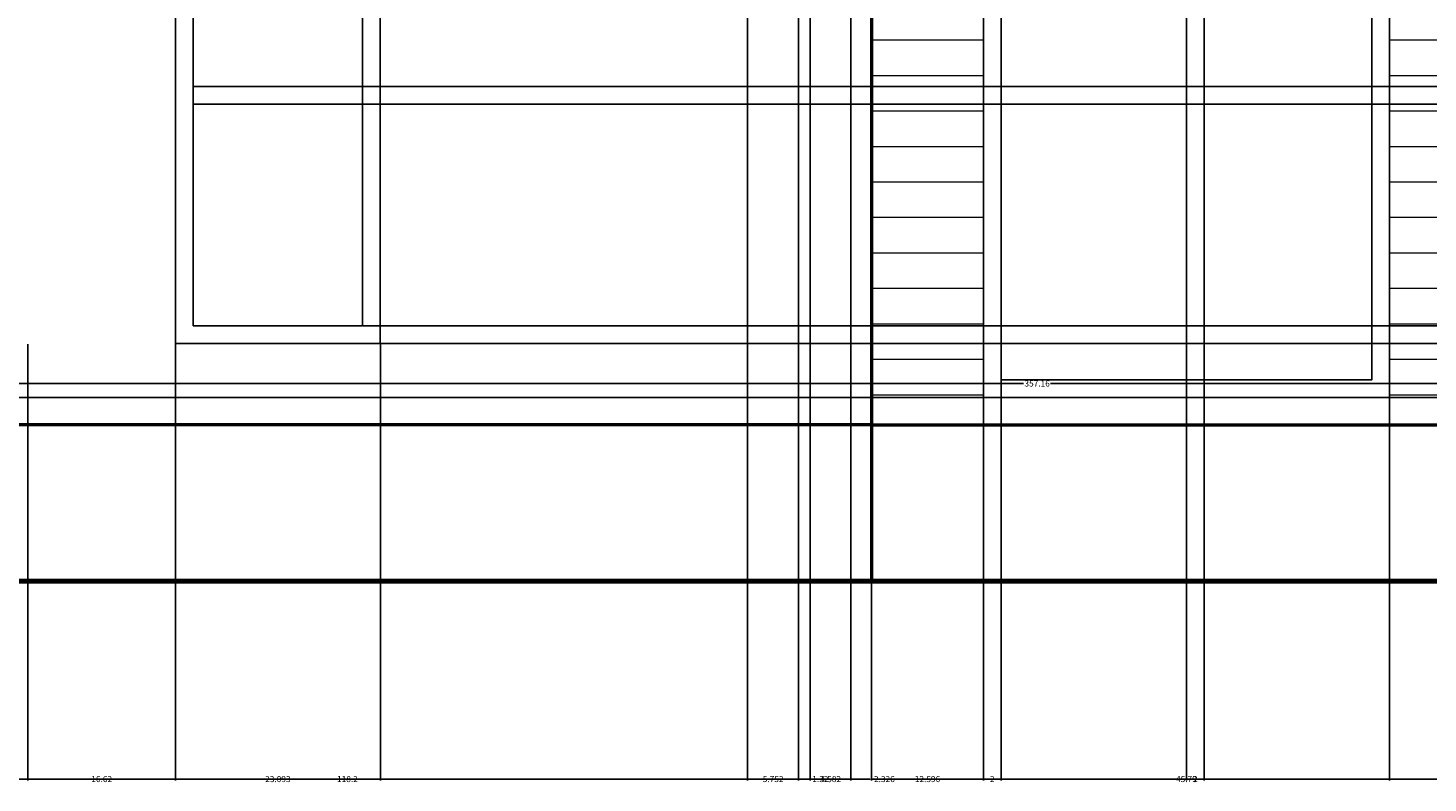
# Model space of a CAD drawing. Units: inches. Extents: x -139 to 346, y 72 to 413.
# Tile 3 of 18: x 18 to 175, y 72 to 157. Entities that reach past the tile are written whole.
import ezdxf

# ---------------------------------------------------------------- set-up
doc = ezdxf.new("R2010")
doc.units = ezdxf.units.IN
doc.header["$MEASUREMENT"] = 0
for name, color, linetype, lineweight in [('A-ANNO-DIMS', 2, 'Continuous', 18), ('A-DOOR', 3, 'Continuous', 25), ('A-GLAZ', 4, 'Continuous', 25), ('A-WALL', 7, 'Continuous', 50), ('A-WALL-PATT', 8, 'Continuous', 13), ('C-TOPO', 7, 'Continuous', 70)]:
    doc.layers.add(name, color=color, linetype=linetype, lineweight=lineweight)
doc.styles.get("Standard").update_dxf_attribs({"font": 'arial.ttf'})
doc.dimstyles.get("Standard").update_dxf_attribs({"dimtxt": 0.6875, "dimasz": 0.18, "dimexe": 0.18, "dimexo": 0.0625, "dimgap": 0.09, "dimtad": 0, "dimtih": 1, "dimtoh": 1, "dimdec": 4, "dimzin": 0, "dimdsep": 46, "dimlunit": 4, "dimtxsty": 'Standard', "dimcen": 0.09, "dimadec": 0, "dimazin": 0, "dimtfac": 1, "dimtdec": 4, "dimtofl": 0, "dimtmove": 0, "dimatfit": 3, "dimfxl": 1, "dimtolj": 1, "dimtzin": 0, "dimarcsym": 0})

# ---------------------------------------------------------------- blocks, each defined once
blk = doc.blocks.new('*D7')
at = {"layer": 'A-ANNO-DIMS', "color": 0, "lineweight": -2, "transparency": 16777216}
for p, q in [((-47.27, 95.04), (-47.27, 117.45)), ((-47.09, 117.27), (129.79, 117.27)), ((309.71, 117.27), (132.82, 117.27)), ((309.89, 95.04), (309.89, 117.45))]:
    blk.add_line(p, q, dxfattribs=at)
at = {"layer": 'A-ANNO-DIMS', "color": 0, "transparency": 16777216}
for points in [[(-47.09, 117.3), (-47.09, 117.24), (-47.27, 117.27)], [(309.71, 117.3), (309.71, 117.24), (309.89, 117.27)]]:
    blk.add_solid(points, dxfattribs=at)
at = {"layer": 'Defpoints', "color": 0, "transparency": 16777216}
for p in [(309.89, 117.27), (-47.27, 94.97), (309.89, 94.97)]:
    blk.add_point(p, dxfattribs=at)
at = {"layer": 'A-ANNO-DIMS', "color": 0, "transparency": 16777216, "insert": (131.31, 117.27), "char_height": 0.688, "attachment_point": 5}
blk.add_mtext('\\A1;357.16', dxfattribs=at)
blk = doc.blocks.new('*D10')
at = {"layer": 'A-ANNO-DIMS', "color": 0, "lineweight": -2, "transparency": 16777216}
for p, q in [((-5.54, 121.71), (-5.54, 72.49)), ((112.65, 112.54), (112.65, 72.49)), ((-5.36, 72.67), (52.34, 72.67)), ((112.47, 72.67), (54.77, 72.67))]:
    blk.add_line(p, q, dxfattribs=at)
at = {"layer": 'A-ANNO-DIMS', "color": 0, "transparency": 16777216}
for points in [[(-5.36, 72.7), (-5.36, 72.64), (-5.54, 72.67)], [(112.47, 72.7), (112.47, 72.64), (112.65, 72.67)]]:
    blk.add_solid(points, dxfattribs=at)
at = {"layer": 'Defpoints', "color": 0, "transparency": 16777216}
for p in [(-5.54, 121.78), (112.65, 112.6), (112.65, 72.67)]:
    blk.add_point(p, dxfattribs=at)
at = {"layer": 'A-ANNO-DIMS', "color": 0, "transparency": 16777216, "insert": (53.56, 72.67), "char_height": 0.688, "attachment_point": 5}
blk.add_mtext('\\A1;118.2', dxfattribs=at)
blk = doc.blocks.new('*D11')
at = {"layer": 'A-ANNO-DIMS', "color": 0, "lineweight": -2, "transparency": 16777216}
for p, q in [((112.65, 112.54), (112.65, 72.49)), ((309.89, 94.91), (309.89, 72.49)), ((112.83, 72.67), (209.79, 72.67)), ((309.71, 72.67), (212.75, 72.67))]:
    blk.add_line(p, q, dxfattribs=at)
at = {"layer": 'A-ANNO-DIMS', "color": 0, "transparency": 16777216}
for points in [[(112.83, 72.7), (112.83, 72.64), (112.65, 72.67)], [(309.71, 72.7), (309.71, 72.64), (309.89, 72.67)]]:
    blk.add_solid(points, dxfattribs=at)
at = {"layer": 'Defpoints', "color": 0, "transparency": 16777216}
for p in [(112.65, 112.6), (309.89, 94.97), (309.89, 72.67)]:
    blk.add_point(p, dxfattribs=at)
at = {"layer": 'A-ANNO-DIMS', "color": 0, "transparency": 16777216, "insert": (211.27, 72.67), "char_height": 0.688, "attachment_point": 5}
blk.add_mtext('\\A1;197.24', dxfattribs=at)
blk = doc.blocks.new('*D12')
at = {"layer": 'A-ANNO-DIMS', "color": 0, "lineweight": -2, "transparency": 16777216}
for p, q in [((-5.54, 121.71), (-5.54, 72.49)), ((17.55, 121.71), (17.55, 72.49)), ((-5.36, 72.67), (4.48, 72.67)), ((17.37, 72.67), (7.53, 72.67))]:
    blk.add_line(p, q, dxfattribs=at)
at = {"layer": 'A-ANNO-DIMS', "color": 0, "transparency": 16777216}
for points in [[(-5.36, 72.7), (-5.36, 72.64), (-5.54, 72.67)], [(17.37, 72.7), (17.37, 72.64), (17.55, 72.67)]]:
    blk.add_solid(points, dxfattribs=at)
at = {"layer": 'Defpoints', "color": 0, "transparency": 16777216}
for p in [(-5.54, 121.78), (17.55, 121.78), (17.55, 72.67)]:
    blk.add_point(p, dxfattribs=at)
at = {"layer": 'A-ANNO-DIMS', "color": 0, "transparency": 16777216, "insert": (6.01, 72.67), "char_height": 0.688, "attachment_point": 5}
blk.add_mtext('\\A1;23.093', dxfattribs=at)
blk = doc.blocks.new('*D13')
at = {"layer": 'A-ANNO-DIMS', "color": 0, "lineweight": -2, "transparency": 16777216}
for p, q in [((17.55, 121.71), (17.55, 72.49)), ((34.17, 121.71), (34.17, 72.49)), ((17.73, 72.67), (24.65, 72.67)), ((33.99, 72.67), (27.08, 72.67))]:
    blk.add_line(p, q, dxfattribs=at)
at = {"layer": 'A-ANNO-DIMS', "color": 0, "transparency": 16777216}
for points in [[(17.73, 72.7), (17.73, 72.64), (17.55, 72.67)], [(33.99, 72.7), (33.99, 72.64), (34.17, 72.67)]]:
    blk.add_solid(points, dxfattribs=at)
at = {"layer": 'Defpoints', "color": 0, "transparency": 16777216}
for p in [(17.55, 121.78), (34.17, 121.78), (34.17, 72.67)]:
    blk.add_point(p, dxfattribs=at)
at = {"layer": 'A-ANNO-DIMS', "color": 0, "transparency": 16777216, "insert": (25.86, 72.67), "char_height": 0.688, "attachment_point": 5}
blk.add_mtext('\\A1;16.62', dxfattribs=at)
blk = doc.blocks.new('*D14')
at = {"layer": 'A-ANNO-DIMS', "color": 0, "lineweight": -2, "transparency": 16777216}
for p, q in [((34.17, 121.71), (34.17, 72.49)), ((57.27, 121.71), (57.27, 72.49)), ((34.35, 72.67), (44.2, 72.67)), ((57.09, 72.67), (47.24, 72.67))]:
    blk.add_line(p, q, dxfattribs=at)
at = {"layer": 'A-ANNO-DIMS', "color": 0, "transparency": 16777216}
for points in [[(34.35, 72.7), (34.35, 72.64), (34.17, 72.67)], [(57.09, 72.7), (57.09, 72.64), (57.27, 72.67)]]:
    blk.add_solid(points, dxfattribs=at)
at = {"layer": 'Defpoints', "color": 0, "transparency": 16777216}
for p in [(34.17, 121.78), (57.27, 121.78), (57.27, 72.67)]:
    blk.add_point(p, dxfattribs=at)
at = {"layer": 'A-ANNO-DIMS', "color": 0, "transparency": 16777216, "insert": (45.72, 72.67), "char_height": 0.688, "attachment_point": 5}
blk.add_mtext('\\A1;23.093', dxfattribs=at)
blk = doc.blocks.new('*D15')
at = {"layer": 'A-ANNO-DIMS', "color": 0, "lineweight": -2, "transparency": 16777216}
for p, q in [((125.25, 115.61), (125.25, 72.49)), ((112.65, 112.54), (112.65, 72.49)), ((112.83, 72.67), (117.46, 72.67)), ((125.07, 72.67), (120.43, 72.67))]:
    blk.add_line(p, q, dxfattribs=at)
at = {"layer": 'A-ANNO-DIMS', "color": 0, "transparency": 16777216}
for points in [[(112.83, 72.7), (112.83, 72.64), (112.65, 72.67)], [(125.07, 72.7), (125.07, 72.64), (125.25, 72.67)]]:
    blk.add_solid(points, dxfattribs=at)
at = {"layer": 'Defpoints', "color": 0, "transparency": 16777216}
for p in [(125.25, 115.68), (112.65, 112.6), (125.25, 72.67)]:
    blk.add_point(p, dxfattribs=at)
at = {"layer": 'A-ANNO-DIMS', "color": 0, "transparency": 16777216, "insert": (118.95, 72.67), "char_height": 0.688, "attachment_point": 5}
blk.add_mtext('\\A1;12.596', dxfattribs=at)
blk = doc.blocks.new('*D16')
at = {"layer": 'A-ANNO-DIMS', "color": 0, "lineweight": -2, "transparency": 16777216}
for p, q in [((125.31, 115.68), (344.39, 115.68)), ((344.21, 115.5), (344.21, 114.58)), ((344.21, 112.78), (344.21, 113.7)), ((112.71, 112.6), (344.39, 112.6))]:
    blk.add_line(p, q, dxfattribs=at)
at = {"layer": 'A-ANNO-DIMS', "color": 0, "transparency": 16777216}
for points in [[(344.18, 115.5), (344.24, 115.5), (344.21, 115.68)], [(344.18, 112.78), (344.24, 112.78), (344.21, 112.6)]]:
    blk.add_solid(points, dxfattribs=at)
at = {"layer": 'Defpoints', "color": 0, "transparency": 16777216}
for p in [(125.25, 115.68), (344.21, 115.68), (112.65, 112.6)]:
    blk.add_point(p, dxfattribs=at)
at = {"layer": 'A-ANNO-DIMS', "color": 0, "transparency": 16777216, "insert": (344.21, 114.14), "char_height": 0.688, "attachment_point": 5}
blk.add_mtext('\\A1;3.072', dxfattribs=at)
blk = doc.blocks.new('*D17')
at = {"layer": 'A-ANNO-DIMS', "color": 0, "lineweight": -2, "transparency": 16777216}
for p, q in [((125.25, 115.61), (125.25, 72.49)), ((171.03, 115.61), (171.03, 72.49)), ((125.43, 72.67), (146.88, 72.67)), ((170.85, 72.67), (149.4, 72.67))]:
    blk.add_line(p, q, dxfattribs=at)
at = {"layer": 'A-ANNO-DIMS', "color": 0, "transparency": 16777216}
for points in [[(125.43, 72.7), (125.43, 72.64), (125.25, 72.67)], [(170.85, 72.7), (170.85, 72.64), (171.03, 72.67)]]:
    blk.add_solid(points, dxfattribs=at)
at = {"layer": 'Defpoints', "color": 0, "transparency": 16777216}
for p in [(125.25, 115.68), (171.03, 115.68), (171.03, 72.67)]:
    blk.add_point(p, dxfattribs=at)
at = {"layer": 'A-ANNO-DIMS', "color": 0, "transparency": 16777216, "insert": (148.14, 72.67), "char_height": 0.688, "attachment_point": 5}
blk.add_mtext('\\A1;45.79', dxfattribs=at)
blk = doc.blocks.new('*D18')
at = {"layer": 'A-ANNO-DIMS', "color": 0, "lineweight": -2, "transparency": 16777216}
for p, q in [((171.03, 115.61), (171.03, 72.49)), ((205.11, 94.91), (205.11, 72.49)), ((171.21, 72.67), (186.82, 72.67)), ((204.93, 72.67), (189.32, 72.67))]:
    blk.add_line(p, q, dxfattribs=at)
at = {"layer": 'A-ANNO-DIMS', "color": 0, "transparency": 16777216}
for points in [[(171.21, 72.7), (171.21, 72.64), (171.03, 72.67)], [(204.93, 72.7), (204.93, 72.64), (205.11, 72.67)]]:
    blk.add_solid(points, dxfattribs=at)
at = {"layer": 'Defpoints', "color": 0, "transparency": 16777216}
for p in [(171.03, 115.68), (205.11, 94.97), (205.11, 72.67)]:
    blk.add_point(p, dxfattribs=at)
at = {"layer": 'A-ANNO-DIMS', "color": 0, "transparency": 16777216, "insert": (188.07, 72.67), "char_height": 0.688, "attachment_point": 5}
blk.add_mtext('\\A1;34.08', dxfattribs=at)
blk = doc.blocks.new('*D62')
at = {"layer": 'A-ANNO-DIMS', "color": 0, "lineweight": -2, "transparency": 16777216}
for p, q in [((55.33, 123.78), (344.39, 123.78)), ((344.21, 123.6), (344.21, 123.21)), ((57.33, 121.78), (344.39, 121.78)), ((344.21, 121.96), (344.21, 122.34))]:
    blk.add_line(p, q, dxfattribs=at)
at = {"layer": 'A-ANNO-DIMS', "color": 0, "transparency": 16777216}
for points in [[(344.18, 123.6), (344.24, 123.6), (344.21, 123.78)], [(344.18, 121.96), (344.24, 121.96), (344.21, 121.78)]]:
    blk.add_solid(points, dxfattribs=at)
at = {"layer": 'Defpoints', "color": 0, "transparency": 16777216}
for p in [(55.27, 123.78), (344.21, 123.78), (57.27, 121.78)]:
    blk.add_point(p, dxfattribs=at)
at = {"layer": 'A-ANNO-DIMS', "color": 0, "transparency": 16777216, "insert": (344.21, 122.78), "char_height": 0.688, "attachment_point": 5}
blk.add_mtext('\\A1;2', dxfattribs=at)
blk = doc.blocks.new('*D63')
at = {"layer": 'A-ANNO-DIMS', "color": 0, "lineweight": -2, "transparency": 16777216}
for p, q in [((55.33, 148.76), (344.39, 148.76)), ((344.21, 148.58), (344.21, 136.71)), ((344.21, 123.96), (344.21, 135.83)), ((55.33, 123.78), (344.39, 123.78))]:
    blk.add_line(p, q, dxfattribs=at)
at = {"layer": 'A-ANNO-DIMS', "color": 0, "transparency": 16777216}
for points in [[(344.18, 148.58), (344.24, 148.58), (344.21, 148.76)], [(344.18, 123.96), (344.24, 123.96), (344.21, 123.78)]]:
    blk.add_solid(points, dxfattribs=at)
at = {"layer": 'Defpoints', "color": 0, "transparency": 16777216}
for p in [(55.27, 148.76), (344.21, 148.76), (55.27, 123.78)]:
    blk.add_point(p, dxfattribs=at)
at = {"layer": 'A-ANNO-DIMS', "color": 0, "transparency": 16777216, "insert": (344.21, 136.27), "char_height": 0.688, "attachment_point": 5}
blk.add_mtext('\\A1;24.98', dxfattribs=at)
blk = doc.blocks.new('*D64')
at = {"layer": 'A-ANNO-DIMS', "color": 0, "lineweight": -2, "transparency": 16777216}
for p, q in [((55.33, 150.76), (344.39, 150.76)), ((344.21, 150.58), (344.21, 150.19)), ((55.33, 148.76), (344.39, 148.76)), ((344.21, 148.94), (344.21, 149.32))]:
    blk.add_line(p, q, dxfattribs=at)
at = {"layer": 'A-ANNO-DIMS', "color": 0, "transparency": 16777216}
for points in [[(344.18, 150.58), (344.24, 150.58), (344.21, 150.76)], [(344.18, 148.94), (344.24, 148.94), (344.21, 148.76)]]:
    blk.add_solid(points, dxfattribs=at)
at = {"layer": 'Defpoints', "color": 0, "transparency": 16777216}
for p in [(55.27, 150.76), (344.21, 150.76), (55.27, 148.76)]:
    blk.add_point(p, dxfattribs=at)
at = {"layer": 'A-ANNO-DIMS', "color": 0, "transparency": 16777216, "insert": (344.21, 149.76), "char_height": 0.688, "attachment_point": 5}
blk.add_mtext('\\A1;2', dxfattribs=at)
blk = doc.blocks.new('*D65')
at = {"layer": 'A-ANNO-DIMS', "color": 0, "lineweight": -2, "transparency": 16777216}
for p, q in [((55.33, 205.52), (344.39, 205.52)), ((344.21, 205.34), (344.21, 178.58)), ((344.21, 150.94), (344.21, 177.7)), ((55.33, 150.76), (344.39, 150.76))]:
    blk.add_line(p, q, dxfattribs=at)
at = {"layer": 'A-ANNO-DIMS', "color": 0, "transparency": 16777216}
for points in [[(344.18, 205.34), (344.24, 205.34), (344.21, 205.52)], [(344.18, 150.94), (344.24, 150.94), (344.21, 150.76)]]:
    blk.add_solid(points, dxfattribs=at)
at = {"layer": 'Defpoints', "color": 0, "transparency": 16777216}
for p in [(55.27, 205.52), (344.21, 205.52), (55.27, 150.76)]:
    blk.add_point(p, dxfattribs=at)
at = {"layer": 'A-ANNO-DIMS', "color": 0, "transparency": 16777216, "insert": (344.21, 178.14), "char_height": 0.688, "attachment_point": 5}
blk.add_mtext('\\A1;54.77', dxfattribs=at)
blk = doc.blocks.new('*D67')
at = {"layer": 'A-ANNO-DIMS', "color": 0, "lineweight": -2, "transparency": 16777216}
for p, q in [((57.33, 207.52), (344.39, 207.52)), ((344.21, 207.34), (344.21, 165.09)), ((344.21, 121.96), (344.21, 164.21)), ((57.33, 121.78), (344.39, 121.78))]:
    blk.add_line(p, q, dxfattribs=at)
at = {"layer": 'A-ANNO-DIMS', "color": 0, "transparency": 16777216}
for points in [[(344.18, 207.34), (344.24, 207.34), (344.21, 207.52)], [(344.18, 121.96), (344.24, 121.96), (344.21, 121.78)]]:
    blk.add_solid(points, dxfattribs=at)
at = {"layer": 'Defpoints', "color": 0, "transparency": 16777216}
for p in [(57.27, 207.52), (344.21, 207.52), (57.27, 121.78)]:
    blk.add_point(p, dxfattribs=at)
at = {"layer": 'A-ANNO-DIMS', "color": 0, "transparency": 16777216, "insert": (344.21, 164.65), "char_height": 0.688, "attachment_point": 5}
blk.add_mtext('\\A1;85.75', dxfattribs=at)
blk = doc.blocks.new('*D70')
at = {"layer": 'A-ANNO-DIMS', "color": 0, "lineweight": -2, "transparency": 16777216}
for p, q in [((125.18, 218.06), (-137.3, 218.06)), ((-137.12, 217.88), (-137.12, 167.31)), ((-137.12, 115.86), (-137.12, 166.43)), ((125.18, 115.68), (-137.3, 115.68))]:
    blk.add_line(p, q, dxfattribs=at)
at = {"layer": 'A-ANNO-DIMS', "color": 0, "transparency": 16777216}
for points in [[(-137.15, 217.88), (-137.09, 217.88), (-137.12, 218.06)], [(-137.15, 115.86), (-137.09, 115.86), (-137.12, 115.68)]]:
    blk.add_solid(points, dxfattribs=at)
at = {"layer": 'Defpoints', "color": 0, "transparency": 16777216}
for p in [(-137.12, 218.06), (125.25, 218.06), (125.25, 115.68)]:
    blk.add_point(p, dxfattribs=at)
at = {"layer": 'A-ANNO-DIMS', "color": 0, "transparency": 16777216, "insert": (-137.12, 166.87), "char_height": 0.688, "attachment_point": 5}
blk.add_mtext('\\A1;102.39', dxfattribs=at)
blk = doc.blocks.new('*D72')
at = {"layer": 'A-ANNO-DIMS', "color": 0, "lineweight": -2, "transparency": 16777216}
for p, q in [((127.25, 117.61), (127.25, 72.49)), ((125.25, 115.61), (125.25, 72.49)), ((125.43, 72.67), (125.93, 72.67)), ((127.07, 72.67), (126.56, 72.67))]:
    blk.add_line(p, q, dxfattribs=at)
at = {"layer": 'A-ANNO-DIMS', "color": 0, "transparency": 16777216}
for points in [[(125.43, 72.7), (125.43, 72.64), (125.25, 72.67)], [(127.07, 72.7), (127.07, 72.64), (127.25, 72.67)]]:
    blk.add_solid(points, dxfattribs=at)
at = {"layer": 'Defpoints', "color": 0, "transparency": 16777216}
for p in [(127.25, 117.68), (125.25, 115.68), (127.25, 72.67)]:
    blk.add_point(p, dxfattribs=at)
at = {"layer": 'A-ANNO-DIMS', "color": 0, "transparency": 16777216, "insert": (126.25, 72.67), "char_height": 0.688, "attachment_point": 5}
blk.add_mtext('\\A1;2', dxfattribs=at)
blk = doc.blocks.new('*D73')
at = {"layer": 'A-ANNO-DIMS', "color": 0, "lineweight": -2, "transparency": 16777216}
for p, q in [((148.14, 117.61), (148.14, 72.49)), ((150.14, 117.61), (150.14, 72.49)), ((148.32, 72.67), (148.82, 72.67)), ((149.96, 72.67), (149.46, 72.67))]:
    blk.add_line(p, q, dxfattribs=at)
at = {"layer": 'A-ANNO-DIMS', "color": 0, "transparency": 16777216}
for points in [[(148.32, 72.7), (148.32, 72.64), (148.14, 72.67)], [(149.96, 72.7), (149.96, 72.64), (150.14, 72.67)]]:
    blk.add_solid(points, dxfattribs=at)
at = {"layer": 'Defpoints', "color": 0, "transparency": 16777216}
for p in [(148.14, 117.68), (150.14, 117.68), (150.14, 72.67)]:
    blk.add_point(p, dxfattribs=at)
at = {"layer": 'A-ANNO-DIMS', "color": 0, "transparency": 16777216, "insert": (149.14, 72.67), "char_height": 0.688, "attachment_point": 5}
blk.add_mtext('\\A1;2', dxfattribs=at)
blk = doc.blocks.new('*D102')
at = {"layer": 'A-ANNO-DIMS', "color": 0, "lineweight": -2, "transparency": 16777216}
for p, q in [((98.67, 291), (98.67, 72.49)), ((104.42, 291), (104.42, 72.49)), ((98.85, 72.67), (100.3, 72.67)), ((104.24, 72.67), (102.79, 72.67))]:
    blk.add_line(p, q, dxfattribs=at)
at = {"layer": 'A-ANNO-DIMS', "color": 0, "transparency": 16777216}
for points in [[(98.85, 72.7), (98.85, 72.64), (98.67, 72.67)], [(104.24, 72.7), (104.24, 72.64), (104.42, 72.67)]]:
    blk.add_solid(points, dxfattribs=at)
at = {"layer": 'Defpoints', "color": 0, "transparency": 16777216}
for p in [(98.67, 291.06), (104.42, 291.06), (104.42, 72.67)]:
    blk.add_point(p, dxfattribs=at)
at = {"layer": 'A-ANNO-DIMS', "color": 0, "transparency": 16777216, "insert": (101.55, 72.67), "char_height": 0.688, "attachment_point": 5}
blk.add_mtext('\\A1;5.752', dxfattribs=at)
blk = doc.blocks.new('*D103')
at = {"layer": 'A-ANNO-DIMS', "color": 0, "lineweight": -2, "transparency": 16777216}
for p, q in [((104.42, 291), (104.42, 72.49)), ((105.74, 291), (105.74, 72.49)), ((104.6, 72.67), (105.56, 72.67)), ((105.74, 72.67), (105.92, 72.67))]:
    blk.add_line(p, q, dxfattribs=at)
at = {"layer": 'A-ANNO-DIMS', "color": 0, "transparency": 16777216}
for points in [[(104.6, 72.7), (104.6, 72.64), (104.42, 72.67)], [(105.56, 72.7), (105.56, 72.64), (105.74, 72.67)]]:
    blk.add_solid(points, dxfattribs=at)
at = {"layer": 'Defpoints', "color": 0, "transparency": 16777216}
for p in [(104.42, 291.06), (105.74, 291.06), (105.74, 72.67)]:
    blk.add_point(p, dxfattribs=at)
at = {"layer": 'A-ANNO-DIMS', "color": 0, "transparency": 16777216, "insert": (106.87, 72.67), "char_height": 0.688, "attachment_point": 5}
blk.add_mtext('\\A1;1.32', dxfattribs=at)
blk = doc.blocks.new('*D104')
at = {"layer": 'A-ANNO-DIMS', "color": 0, "lineweight": -2, "transparency": 16777216}
for p, q in [((110.32, 298.23), (110.32, 72.49)), ((105.74, 291), (105.74, 72.49)), ((105.92, 72.67), (106.77, 72.67)), ((110.14, 72.67), (109.29, 72.67))]:
    blk.add_line(p, q, dxfattribs=at)
at = {"layer": 'A-ANNO-DIMS', "color": 0, "transparency": 16777216}
for points in [[(105.92, 72.7), (105.92, 72.64), (105.74, 72.67)], [(110.14, 72.7), (110.14, 72.64), (110.32, 72.67)]]:
    blk.add_solid(points, dxfattribs=at)
at = {"layer": 'Defpoints', "color": 0, "transparency": 16777216}
for p in [(110.32, 298.29), (105.74, 291.06), (110.32, 72.67)]:
    blk.add_point(p, dxfattribs=at)
at = {"layer": 'A-ANNO-DIMS', "color": 0, "transparency": 16777216, "insert": (108.03, 72.67), "char_height": 0.688, "attachment_point": 5}
blk.add_mtext('\\A1;4.582', dxfattribs=at)
blk = doc.blocks.new('*D105')
at = {"layer": 'A-ANNO-DIMS', "color": 0, "lineweight": -2, "transparency": 16777216}
for p, q in [((110.32, 298.23), (110.32, 72.49)), ((112.65, 289), (112.65, 72.49)), ((110.5, 72.67), (112.47, 72.67)), ((112.65, 72.67), (112.83, 72.67))]:
    blk.add_line(p, q, dxfattribs=at)
at = {"layer": 'A-ANNO-DIMS', "color": 0, "transparency": 16777216}
for points in [[(110.5, 72.7), (110.5, 72.64), (110.32, 72.67)], [(112.47, 72.7), (112.47, 72.64), (112.65, 72.67)]]:
    blk.add_solid(points, dxfattribs=at)
at = {"layer": 'Defpoints', "color": 0, "transparency": 16777216}
for p in [(110.32, 298.29), (112.65, 289.06), (112.65, 72.67)]:
    blk.add_point(p, dxfattribs=at)
at = {"layer": 'A-ANNO-DIMS', "color": 0, "transparency": 16777216, "insert": (114.09, 72.67), "char_height": 0.688, "attachment_point": 5}
blk.add_mtext('\\A1;2.326', dxfattribs=at)

msp = doc.modelspace()

# ---------------------------------------------------------------- hatches: boundary and pattern name
at = {"layer": 'A-WALL-PATT'}
h = msp.add_hatch(dxfattribs=at)
h.set_pattern_fill('ANSI31', color=256, scale=32, angle=135)
h.paths.add_polyline_path([(98.6724, 360.5443), (-34.7346, 360.5443), (-34.7346, 353.0644), (-34.7346, 305.9205), (5.6729, 305.9205), (5.6729, 338.3217), (62.4258, 338.3217), (62.4258, 305.9205), (98.6724, 305.9205)])
h.paths.add_polyline_path([(212.769, 231.0607), (175.072, 231.0607), (175.072, 218.0635), (171.0337, 218.0635), (171.0337, 115.6761), (125.2464, 115.6761), (125.2464, 218.0635), (123.4318, 218.0635), (120.5054, 218.0635), (120.5054, 231.0607), (112.6506, 231.0607), (112.6506, 112.6042), (212.769, 112.6042)])

# ---------------------------------------------------------------- linework, layer by layer
at = {"layer": 'A-DOOR'}
for p, q in [((148.1401, 212.5413), (148.1401, 117.6761)), ((150.1401, 212.5413), (150.1401, 117.6761))]:
    msp.add_line(p, q, dxfattribs=at)
for points in [[(125.2464, 218.0635), (171.0337, 218.0635), (171.0337, 115.6761), (125.2464, 115.6761)], [(127.2464, 216.0635), (169.0337, 216.0635), (169.0337, 117.6761), (127.2464, 117.6761)]]:
    msp.add_lwpolyline(points, close=True, dxfattribs=at)
at = {"layer": 'A-GLAZ'}
for p, q in [((36.1727, 150.7576), (55.2654, 150.7576)), ((36.1727, 148.7576), (55.2654, 148.7576))]:
    msp.add_line(p, q, dxfattribs=at)
for points in [[(34.1727, 207.5243), (57.2654, 207.5243), (57.2654, 121.7753), (34.1727, 121.7753)], [(36.1727, 205.5243), (55.2654, 205.5243), (55.2654, 123.7753), (36.1727, 123.7753)]]:
    msp.add_lwpolyline(points, close=True, dxfattribs=at)
at = {"layer": 'A-WALL'}
for p, q in [((112.6506, 238.9748), (112.6506, 94.9748)), ((112.6506, 112.6042), (-47.2734, 112.6042)), ((112.6506, 112.6042), (297.5013, 112.6042))]:
    msp.add_line(p, q, dxfattribs=at)
at = {"layer": 'C-TOPO'}
for p, q in [((-47.2734, 94.9748), (51.0187, 94.9748)), ((51.0187, 94.9748), (321.9055, 94.9748))]:
    msp.add_line(p, q, dxfattribs=at)

# ---------------------------------------------------------------- dimensions: what is measured, and where the dimension line sits
at = {"layer": 'A-ANNO-DIMS'}
for base, p1, p2, override, picture, middle in [((110.3243, 72.6748), (105.7421, 291.0604), (110.3243, 298.293), {"dimdec": 3, "dimlfac": 1, "dimrnd": 0, "dimzin": 0, "dimdsep": 46, "dimlunit": 2}, '*D104', (108.0332, 72.6748)), ((112.6506, 72.6748), (110.3243, 298.293), (112.6506, 289.0604), {"dimdec": 3, "dimlfac": 1, "dimrnd": 0, "dimzin": 0, "dimdsep": 46, "dimlunit": 2}, '*D105', (114.0862, 72.6748)), ((104.4244, 72.6748), (98.6724, 291.0604), (104.4244, 291.0604), {"dimdec": 3, "dimlfac": 1, "dimrnd": 0, "dimzin": 0, "dimdsep": 46, "dimlunit": 2}, '*D102', (101.5484, 72.6748)), ((105.7421, 72.6748), (104.4244, 291.0604), (105.7421, 291.0604), {"dimdec": 2, "dimlfac": 1, "dimrnd": 0, "dimzin": 0, "dimdsep": 46, "dimlunit": 2}, '*D103', (106.8691, 72.6748)), ((112.6506, 72.6748), (-5.5402, 121.7753), (112.6506, 112.6042), {"dimdec": 1, "dimlfac": 1, "dimrnd": 0, "dimzin": 0, "dimdsep": 46, "dimlunit": 2}, '*D10', (53.5552, 72.6748)), ((17.5525, 72.6748), (-5.5402, 121.7753), (17.5525, 121.7753), {"dimdec": 3, "dimlfac": 1, "dimrnd": 0, "dimzin": 0, "dimdsep": 46, "dimlunit": 2}, '*D12', (6.0062, 72.6748)), ((34.1727, 72.6748), (17.5525, 121.7753), (34.1727, 121.7753), {"dimdec": 2, "dimlfac": 1, "dimrnd": 0, "dimzin": 0, "dimdsep": 46, "dimlunit": 2}, '*D13', (25.8626, 72.6748)), ((57.2654, 72.6748), (34.1727, 121.7753), (57.2654, 121.7753), {"dimdec": 3, "dimlfac": 1, "dimrnd": 0, "dimzin": 0, "dimdsep": 46, "dimlunit": 2}, '*D14', (45.719, 72.6748)), ((309.8894, 117.2748), (-47.2734, 94.9748), (309.8894, 94.9748), {"dimdec": 2, "dimlfac": 1, "dimrnd": 0, "dimzin": 0, "dimdsep": 46, "dimlunit": 2}, '*D7', (131.308, 117.2748)), ((127.2464, 72.6748), (125.2464, 115.6761), (127.2464, 117.6761), {"dimdec": 0, "dimlfac": 1, "dimrnd": 0, "dimzin": 0, "dimdsep": 46, "dimlunit": 2}, '*D72', (126.2464, 72.6748)), ((150.1401, 72.6748), (148.1401, 117.6761), (150.1401, 117.6761), {"dimdec": 0, "dimlfac": 1, "dimrnd": 0, "dimzin": 0, "dimdsep": 46, "dimlunit": 2}, '*D73', (149.1401, 72.6748)), ((125.2464, 72.6748), (112.6506, 112.6042), (125.2464, 115.6761), {"dimdec": 3, "dimlfac": 1, "dimrnd": 0, "dimzin": 0, "dimdsep": 46, "dimlunit": 2}, '*D15', (118.9485, 72.6748)), ((171.0337, 72.6748), (125.2464, 115.6761), (171.0337, 115.6761), {"dimdec": 2, "dimlfac": 1, "dimrnd": 0, "dimzin": 0, "dimdsep": 46, "dimlunit": 2}, '*D17', (148.1401, 72.6748)), ((205.1121, 72.6748), (171.0337, 115.6761), (205.1121, 94.9748), {"dimdec": 2, "dimlfac": 1, "dimrnd": 0, "dimzin": 0, "dimdsep": 46, "dimlunit": 2}, '*D18', (188.0729, 72.6748)), ((309.8894, 72.6748), (112.6506, 112.6042), (309.8894, 94.9748), {"dimdec": 2, "dimlfac": 1, "dimrnd": 0, "dimzin": 0, "dimdsep": 46, "dimlunit": 2}, '*D11', (211.27, 72.6748))]:
    dim = msp.add_linear_dim(base=base, p1=p1, p2=p2, dimstyle='Standard', override=override, dxfattribs=at)
    dim.commit()
    dim.dimension.update_dxf_attribs({"geometry": picture, "text_midpoint": middle})
for base, p1, p2, override, picture, middle in [((-137.1237, 218.0635), (125.2464, 115.6761), (125.2464, 218.0635), {"dimdec": 2, "dimlfac": 1, "dimrnd": 0, "dimzin": 0, "dimdsep": 46, "dimlunit": 2}, '*D70', (-137.1237, 166.8698)), ((344.2055, 207.5243), (57.2654, 121.7753), (57.2654, 207.5243), {"dimdec": 2, "dimlfac": 1, "dimrnd": 0, "dimzin": 0, "dimdsep": 46, "dimlunit": 2}, '*D67', (344.2055, 164.6498)), ((344.2055, 205.5243), (55.2654, 150.7576), (55.2654, 205.5243), {"dimdec": 2, "dimlfac": 1, "dimrnd": 0, "dimzin": 0, "dimdsep": 46, "dimlunit": 2}, '*D65', (344.2055, 178.141)), ((344.2055, 150.7576), (55.2654, 148.7576), (55.2654, 150.7576), {"dimdec": 0, "dimlfac": 1, "dimrnd": 0, "dimzin": 0, "dimdsep": 46, "dimlunit": 2}, '*D64', (344.2055, 149.7576)), ((344.2055, 148.7576), (55.2654, 123.7753), (55.2654, 148.7576), {"dimdec": 2, "dimlfac": 1, "dimrnd": 0, "dimzin": 0, "dimdsep": 46, "dimlunit": 2}, '*D63', (344.2055, 136.2665)), ((344.2055, 123.7753), (57.2654, 121.7753), (55.2654, 123.7753), {"dimdec": 0, "dimlfac": 1, "dimrnd": 0, "dimzin": 0, "dimdsep": 46, "dimlunit": 2}, '*D62', (344.2055, 122.7753)), ((344.2055, 115.6761), (112.6506, 112.6042), (125.2464, 115.6761), {"dimdec": 3, "dimlfac": 1, "dimrnd": 0, "dimzin": 0, "dimdsep": 46, "dimlunit": 2}, '*D16', (344.2055, 114.1402))]:
    dim = msp.add_linear_dim(base=base, p1=p1, p2=p2, angle=90, dimstyle='Standard', override=override, dxfattribs=at)
    dim.commit()
    dim.dimension.update_dxf_attribs({"geometry": picture, "text_midpoint": middle})

doc.saveas('drawing.dxf')
